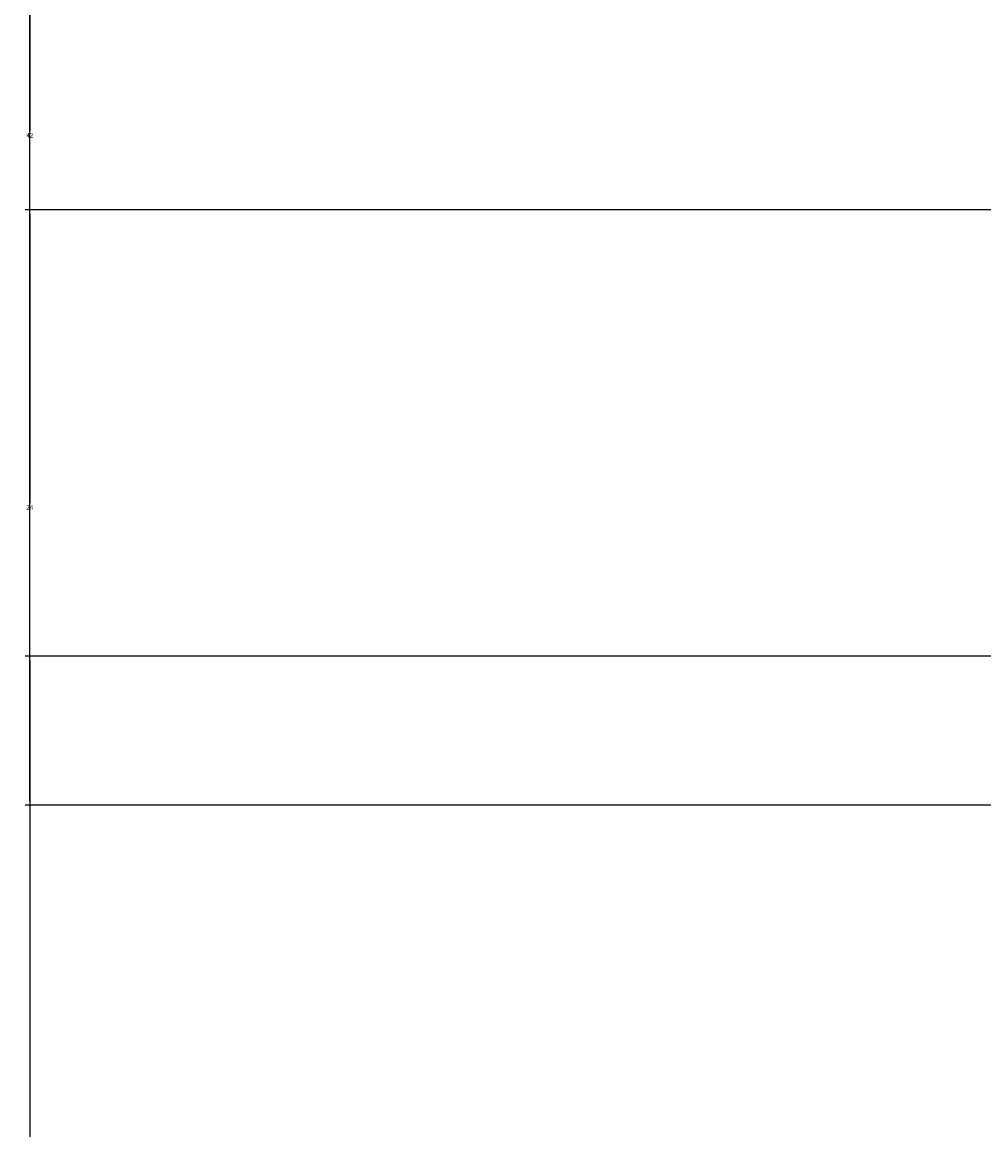
# Model space of a CAD drawing. Units: inches. Extents: x 1998 to 2588, y 1139 to 1977.
# Tile 3 of 134: x 1998 to 2036, y 1576 to 1620. Entities that reach past the tile are written whole.
import ezdxf

# ---------------------------------------------------------------- set-up
doc = ezdxf.new("R2010")
doc.units = ezdxf.units.IN
doc.layers.add('A-ANNO-DIMS', color=2, linetype='Continuous', lineweight=18)
doc.styles.get("Standard").update_dxf_attribs({"font": 'arial.ttf'})
doc.dimstyles.get("Standard").update_dxf_attribs({"dimtxt": 0.18, "dimasz": 0.18, "dimexe": 0.18, "dimexo": 0.0625, "dimgap": 0.09, "dimtad": 0, "dimtih": 1, "dimtoh": 1, "dimdec": 4, "dimzin": 0, "dimdsep": 46, "dimtxsty": 'Standard', "dimcen": 0.09, "dimadec": 0, "dimazin": 0, "dimtfac": 1, "dimtdec": 4, "dimtofl": 0, "dimtmove": 0, "dimatfit": 3, "dimfxl": 1, "dimtolj": 1, "dimtzin": 0, "dimarcsym": 0})

# ---------------------------------------------------------------- blocks, each defined once
blk = doc.blocks.new('*D30')
at = {"layer": 'A-ANNO-DIMS', "color": 0, "lineweight": -2, "transparency": 16777216}
for p, q in [((2407.91, 1636.732), (1997.843, 1636.732)), ((1998.023, 1636.552), (1998.023, 1615.913)), ((1998.023, 1594.912), (1998.023, 1615.552)), ((2407.91, 1594.732), (1997.843, 1594.732))]:
    blk.add_line(p, q, dxfattribs=at)
at = {"layer": 'A-ANNO-DIMS', "color": 0, "transparency": 16777216}
for points in [[(1997.993, 1636.552), (1998.053, 1636.552), (1998.023, 1636.732)], [(1997.993, 1594.912), (1998.053, 1594.912), (1998.023, 1594.732)]]:
    blk.add_solid(points, dxfattribs=at)
at = {"layer": 'Defpoints', "color": 0, "transparency": 16777216}
for p in [(1998.023, 1636.732), (2407.973, 1636.732), (2407.973, 1594.732)]:
    blk.add_point(p, dxfattribs=at)
at = {"layer": 'A-ANNO-DIMS', "color": 0, "transparency": 16777216, "insert": (1998.023, 1615.732), "char_height": 0.18, "attachment_point": 5}
blk.add_mtext('\\A1;42', dxfattribs=at)
blk = doc.blocks.new('*D34')
at = {"layer": 'A-ANNO-DIMS', "color": 0, "lineweight": -2, "transparency": 16777216}
for p, q in [((2407.91, 1594.732), (1997.843, 1594.732)), ((1998.023, 1594.552), (1998.023, 1558.913)), ((1998.023, 1522.912), (1998.023, 1558.552)), ((2407.91, 1522.732), (1997.843, 1522.732))]:
    blk.add_line(p, q, dxfattribs=at)
at = {"layer": 'A-ANNO-DIMS', "color": 0, "transparency": 16777216}
for points in [[(1997.993, 1594.552), (1998.053, 1594.552), (1998.023, 1594.732)], [(1997.993, 1522.912), (1998.053, 1522.912), (1998.023, 1522.732)]]:
    blk.add_solid(points, dxfattribs=at)
at = {"layer": 'Defpoints', "color": 0, "transparency": 16777216}
for p in [(1998.023, 1594.732), (2407.973, 1594.732), (2407.973, 1522.732)]:
    blk.add_point(p, dxfattribs=at)
at = {"layer": 'A-ANNO-DIMS', "color": 0, "transparency": 16777216, "insert": (1998.023, 1558.732), "char_height": 0.18, "attachment_point": 5}
blk.add_mtext('\\A1;72', dxfattribs=at)
blk = doc.blocks.new('*D35')
at = {"layer": 'A-ANNO-DIMS', "color": 0, "lineweight": -2, "transparency": 16777216}
for p, q in [((2148.392, 1612.732), (1997.843, 1612.732)), ((1998.023, 1612.552), (1998.023, 1600.913)), ((1998.023, 1588.912), (1998.023, 1600.552)), ((2148.392, 1588.732), (1997.843, 1588.732))]:
    blk.add_line(p, q, dxfattribs=at)
at = {"layer": 'A-ANNO-DIMS', "color": 0, "transparency": 16777216}
for points in [[(1997.993, 1612.552), (1998.053, 1612.552), (1998.023, 1612.732)], [(1997.993, 1588.912), (1998.053, 1588.912), (1998.023, 1588.732)]]:
    blk.add_solid(points, dxfattribs=at)
at = {"layer": 'Defpoints', "color": 0, "transparency": 16777216}
for p in [(1998.023, 1612.732), (2148.455, 1612.732), (2148.455, 1588.732)]:
    blk.add_point(p, dxfattribs=at)
at = {"layer": 'A-ANNO-DIMS', "color": 0, "transparency": 16777216, "insert": (1998.023, 1600.732), "char_height": 0.18, "attachment_point": 5}
blk.add_mtext('\\A1;24', dxfattribs=at)
blk = doc.blocks.new('*D38')
at = {"layer": 'A-ANNO-DIMS', "color": 0, "lineweight": -2, "transparency": 16777216}
for p, q in [((2197.387, 1663.247), (1997.843, 1663.247)), ((1998.023, 1663.067), (1998.023, 1638.171)), ((1998.023, 1612.912), (1998.023, 1637.808)), ((2197.387, 1612.732), (1997.843, 1612.732))]:
    blk.add_line(p, q, dxfattribs=at)
at = {"layer": 'A-ANNO-DIMS', "color": 0, "transparency": 16777216}
for points in [[(1997.993, 1663.067), (1998.053, 1663.067), (1998.023, 1663.247)], [(1997.993, 1612.912), (1998.053, 1612.912), (1998.023, 1612.732)]]:
    blk.add_solid(points, dxfattribs=at)
at = {"layer": 'Defpoints', "color": 0, "transparency": 16777216}
for p in [(1998.023, 1663.247), (2197.45, 1663.247), (2197.45, 1612.732)]:
    blk.add_point(p, dxfattribs=at)
at = {"layer": 'A-ANNO-DIMS', "color": 0, "transparency": 16777216, "insert": (1998.023, 1637.99), "char_height": 0.18, "attachment_point": 5}
blk.add_mtext('\\A1;50.51', dxfattribs=at)

msp = doc.modelspace()

# ---------------------------------------------------------------- dimensions: what is measured, and where the dimension line sits
at = {"layer": 'A-ANNO-DIMS'}
for base, p1, p2, override, picture, middle in [((1998.0229, 1663.2466), (2197.4499, 1612.7324), (2197.4499, 1663.2466), {"dimdec": 2, "dimlfac": 1, "dimrnd": 0, "dimzin": 0, "dimdsep": 46, "dimlunit": 2}, '*D38', (1998.0229, 1637.9895)), ((1998.0229, 1636.7324), (2407.9729, 1594.7324), (2407.9729, 1636.7324), {"dimdec": 0, "dimlfac": 1, "dimrnd": 0, "dimzin": 0, "dimdsep": 46, "dimlunit": 2}, '*D30', (1998.0229, 1615.7324)), ((1998.0229, 1612.7324), (2148.4548, 1588.7324), (2148.4548, 1612.7324), {"dimdec": 0, "dimlfac": 1, "dimrnd": 0, "dimzin": 0, "dimdsep": 46, "dimlunit": 2}, '*D35', (1998.0229, 1600.7324)), ((1998.0229, 1594.7324), (2407.9729, 1522.7324), (2407.9729, 1594.7324), {"dimdec": 0, "dimlfac": 1, "dimrnd": 0, "dimzin": 0, "dimdsep": 46, "dimlunit": 2}, '*D34', (1998.0229, 1558.7324))]:
    dim = msp.add_linear_dim(base=base, p1=p1, p2=p2, angle=90, dimstyle='Standard', override=override, dxfattribs=at)
    dim.commit()
    dim.dimension.update_dxf_attribs({"geometry": picture, "text_midpoint": middle})

doc.saveas('drawing.dxf')
